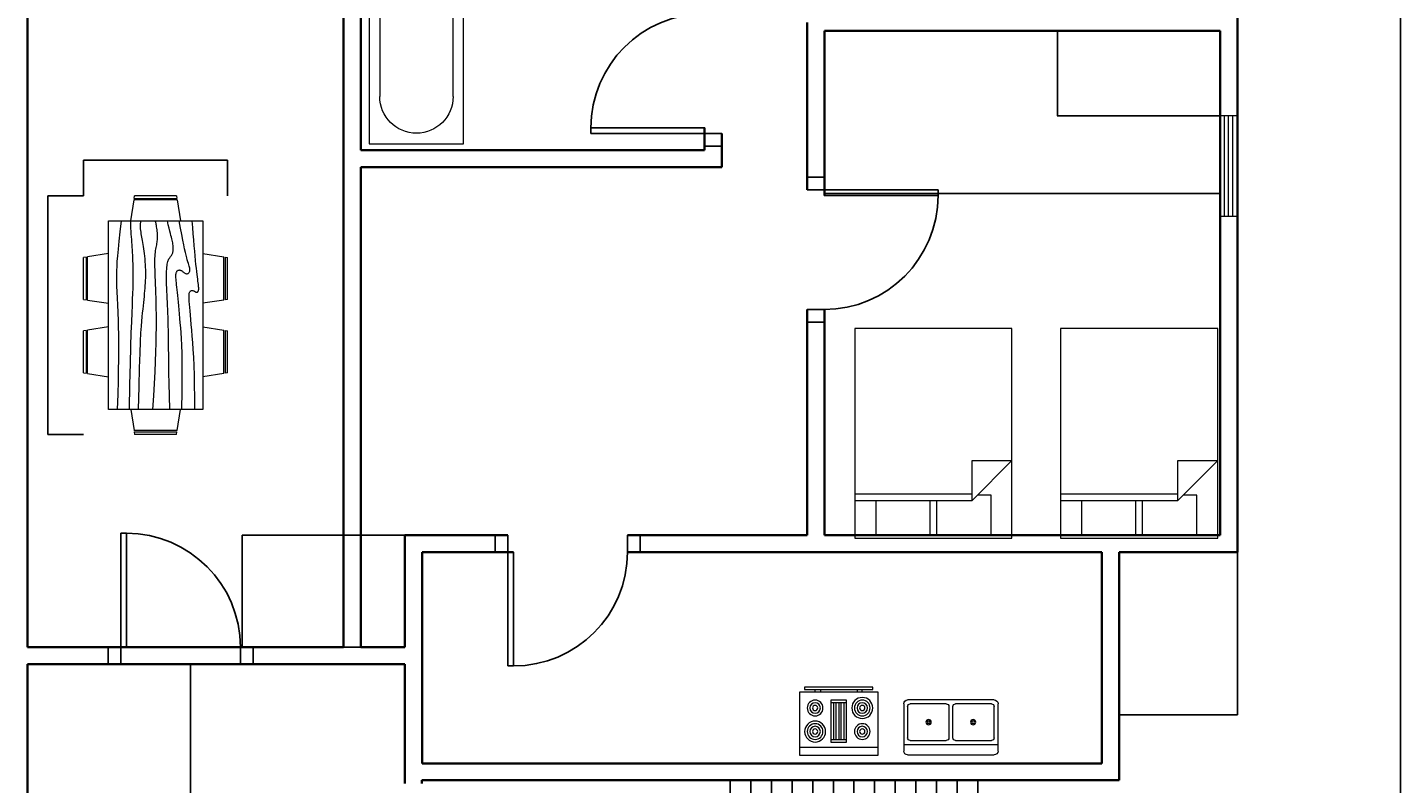
# Model space of a CAD drawing. Units: millimetres. Extents: x 31 to 27050, y -916 to 32407.
# Tile 7 of 7: x 13741 to 27050, y 16782 to 24108. Entities that reach past the tile are written whole.
import ezdxf

# ---------------------------------------------------------------- set-up
doc = ezdxf.new("R2010")
doc.units = ezdxf.units.MM
for name, color, linetype, lineweight in [('A-ANNO-DIMS', 2, 'Continuous', 18), ('A-DOOR', 3, 'Continuous', 25), ('A-EQPM', 8, 'Continuous', 18), ('A-FLOR-FIXT', 9, 'Continuous', 18), ('A-FLOR-STRS', 7, 'Continuous', 25), ('A-FURN', 8, 'Continuous', 13), ('A-GLAZ', 4, 'Continuous', 18), ('A-WALL', 7, 'Continuous', 35)]:
    doc.layers.add(name, color=color, linetype=linetype, lineweight=lineweight)
doc.styles.get("Standard").update_dxf_attribs({"font": 'arial.ttf'})
doc.dimstyles.get("Standard").update_dxf_attribs({"dimtxt": 0.18, "dimasz": 0.18, "dimexe": 0.18, "dimexo": 0.0625, "dimgap": 0.09, "dimtad": 0, "dimtih": 1, "dimtoh": 1, "dimdec": 4, "dimzin": 0, "dimdsep": 46, "dimtxsty": 'Standard', "dimcen": 0.09, "dimadec": 0, "dimazin": 0, "dimtfac": 1, "dimtdec": 4, "dimtofl": 0, "dimtmove": 0, "dimatfit": 3, "dimfxl": 1, "dimtolj": 1, "dimtzin": 0, "dimarcsym": 0})

# ---------------------------------------------------------------- blocks, each defined once
blk = doc.blocks.new('Dining Set - 36 x 72 in.')
for p, q in [((-22, 27.5), (-22.15620000000001, 26.50042)), ((-5.841600000000028, 26.5), (-22.15340000000003, 26.5)), ((-22, 27.5), (-6, 27.5)), ((-5.843700000000012, 26.49966), (-6, 27.5)), ((6, 27.5), (5.843799999999987, 26.50042)), ((22.15839999999997, 26.5), (5.846599999999966, 26.5)), ((6, 27.5), (22, 27.5)), ((22.15629999999999, 26.49966), (22, 27.5)), ((-22.23430000000002, 26.00059), (-23.48470000000003, 17.99762)), ((-22.23040000000003, 26), (-5.760800000000017, 26)), ((-4.515199999999992, 17.99762), (-5.765500000000031, 25.99926)), ((5.765699999999981, 26.00059), (4.515299999999967, 17.99762)), ((5.769599999999968, 26), (22.23919999999998, 26)), ((23.48480000000001, 17.99762), (22.23449999999997, 25.99926)), ((36, 18), (-36, 18)), ((-36, 18), (-36, -18)), ((36, -18), (36, 18)), ((-45.49999999999999, 8.000000000000004), (-44.50040000000001, 8.156170000000007)), ((-45.49999999999999, 8.000000000000004), (-45.49999999999999, -7.999999999999996)), ((-44.5, -8.15843), (-44.5, 8.153380000000002)), ((-44.00060000000002, 8.234280000000002), (-35.99760000000003, 9.484740000000006)), ((-44, 8.230410000000003), (-44, -8.239149999999999)), ((44.00059999999996, 8.234280000000002), (35.99759999999998, 9.484740000000006)), ((44, 8.230410000000003), (44, -8.239149999999999)), ((44.5, -8.15843), (44.5, 8.153380000000002)), ((45.49999999999999, 8.000000000000004), (44.50049999999999, 8.156170000000007)), ((45.49999999999999, 8.000000000000004), (45.49999999999999, -7.999999999999996)), ((-44.49970000000002, -8.156309999999994), (-45.49999999999999, -7.999999999999996)), ((-35.99760000000003, -9.484759999999998), (-43.9993, -8.234499999999993)), ((35.99759999999998, -9.484759999999998), (43.9993, -8.234499999999993)), ((44.49969999999995, -8.156309999999994), (45.49999999999999, -7.999999999999996)), ((-36, -18), (36, -18)), ((-22.23430000000002, -26.0006), (-23.48470000000003, -17.99762)), ((-4.515199999999992, -17.99762), (-5.765500000000031, -25.99928)), ((5.765699999999981, -26.0006), (4.515299999999967, -17.99762)), ((23.48480000000001, -17.99762), (22.23449999999997, -25.99928)), ((-22.23040000000003, -26), (-5.760800000000017, -26)), ((5.769599999999968, -26), (22.23919999999998, -26)), ((-22, -27.5), (-22.15620000000001, -26.50044)), ((-5.841600000000028, -26.5), (-22.15340000000003, -26.5)), ((-22, -27.5), (-6, -27.5)), ((-5.843700000000012, -26.49967), (-6, -27.5)), ((6, -27.5), (5.843799999999987, -26.50044)), ((22.15839999999997, -26.5), (5.846599999999966, -26.5)), ((6, -27.5), (22, -27.5)), ((22.15629999999999, -26.49967), (22, -27.5))]:
    blk.add_line(p, q)
for points in [[(-36, 15), (-31.17720000000003, 14.97754), (-26.80790000000002, 14.91406), (-22.85380000000003, 14.81543), (-19.27600000000001, 14.6875), (-16.03620000000001, 14.53613), (-13.09570000000002, 14.36718), (-10.41590000000002, 14.18652), (-7.958300000000008, 14), (-5.690400000000011, 13.81315), (-3.603499999999996, 13.63021), (-1.695400000000006, 13.45508), (0.0364999999999896, 13.29166), (1.594499999999982, 13.14388), (2.981099999999969, 13.01562), (4.198800000000005, 12.9108), (5.25, 12.83333), (6.139299999999991, 12.78613), (6.880200000000002, 12.76823), (7.488299999999981, 12.77767), (7.979199999999991, 12.8125), (8.368499999999983, 12.87077), (8.671899999999994, 12.95052), (8.904899999999998, 13.0498), (9.083300000000008, 13.16666), (9.220499999999959, 13.29899000000001), (9.32159999999999, 13.44401), (9.389499999999998, 13.59879), (9.427099999999996, 13.76041), (9.437299999999993, 13.92594), (9.423200000000008, 14.09245), (9.387499999999989, 14.257), (9.333300000000008, 14.41666), (9.263800000000003, 14.56917), (9.183600000000013, 14.71484), (9.097499999999968, 14.85465), (9.010400000000004, 14.98958), (8.92719999999997, 15.12060000000001), (8.852899999999975, 15.2487), (8.79219999999998, 15.37483), (8.75, 15.5), (8.730500000000006, 15.62467), (8.734399999999994, 15.74739), (8.761699999999962, 15.86621), (8.8125, 15.97916), (8.886699999999962, 16.08431), (8.984399999999994, 16.17968), (9.105500000000006, 16.26334), (9.25, 16.33333), (9.418900000000008, 16.38802), (9.617199999999968, 16.42708), (9.850599999999986, 16.45052), (10.125, 16.45833), (10.44630000000001, 16.45052), (10.82029999999997, 16.42708), (11.25290000000001, 16.38802), (11.75, 16.33333), (12.3184, 16.26318), (12.96940000000001, 16.17838), (13.7151, 16.07991), (14.5677, 15.96875), (15.53949999999997, 15.84586), (16.64259999999996, 15.71224), (17.88929999999999, 15.56884), (19.29169999999999, 15.41666), (20.85899999999998, 15.25667), (22.58789999999999, 15.08984), (24.47210000000001, 14.91715), (26.5052, 14.73958), (28.68090000000001, 14.5581), (30.99289999999996, 14.3737), (33.43469999999996, 14.18733), (36, 14)], [(-36, 10), (-28.97660000000002, 10.14274000000001), (-23.17250000000001, 10.20442), (-18.42410000000001, 10.19775), (-14.5677, 10.13541), (-11.43990000000002, 10.03011), (-8.87700000000001, 9.894530000000007), (-6.715399999999988, 9.741370000000005), (-4.791699999999991, 9.58333), (-2.96980000000002, 9.43082), (-1.224600000000009, 9.285150000000005), (0.4414999999999623, 9.14534), (2.02600000000001, 9.010410000000004), (3.526599999999973, 8.879390000000004), (4.940799999999967, 8.751300000000004), (6.265999999999962, 8.625160000000005), (7.5, 8.500000000000004), (8.641099999999994, 8.375490000000003), (9.691399999999987, 8.253900000000005), (10.65379999999999, 8.13818), (11.53120000000001, 8.031250000000004), (12.32669999999996, 7.936030000000005), (13.043, 7.85547), (13.68309999999997, 7.792480000000001), (14.25, 7.750000000000003), (14.74709999999999, 7.730300000000003), (15.17969999999997, 7.733070000000001), (15.55369999999999, 7.757320000000003), (15.875, 7.80208), (16.14940000000001, 7.866370000000006), (16.38279999999997, 7.94922), (16.58109999999999, 8.04964), (16.75, 8.166660000000004), (16.89439999999996, 8.29915), (17.01429999999999, 8.445310000000003), (17.1089, 8.603190000000001), (17.17709999999999, 8.77083), (17.21799999999996, 8.946290000000001), (17.2305, 9.127600000000005), (17.21369999999996, 9.312820000000006), (17.16669999999999, 9.500000000000004), (17.08949999999999, 9.687500000000004), (16.98699999999996, 9.875000000000004), (16.86489999999998, 10.0625), (16.72919999999999, 10.25), (16.5856, 10.4375), (16.44009999999997, 10.625), (16.29849999999999, 10.8125), (16.16669999999999, 11), (16.05000000000001, 11.18733), (15.95179999999999, 11.3737), (15.8752, 11.5581), (15.8229, 11.73958), (15.798, 11.91715), (15.80340000000001, 12.08984), (15.84199999999998, 12.25667), (15.91669999999999, 12.41666), (16.02949999999998, 12.56836), (16.17840000000001, 12.70833), (16.3605, 12.83268), (16.5729, 12.9375), (16.8127, 13.01888000000001), (17.07679999999999, 13.07291), (17.36250000000001, 13.0957), (17.66669999999999, 13.08333), (17.98939999999999, 13.03312), (18.34179999999998, 12.94726), (18.7382, 12.82918), (19.1927, 12.68229), (19.71949999999998, 12.51001), (20.33269999999999, 12.31575), (21.04649999999998, 12.10294), (21.875, 11.875), (22.83569999999997, 11.63354), (23.95900000000001, 11.37304), (25.27859999999999, 11.08618), (26.82819999999998, 10.76562), (28.64139999999998, 10.40405), (30.75200000000001, 9.994140000000005), (33.1936, 9.528560000000002), (36, 9.000000000000004)], [(-36, 5.500000000000003), (-30.71570000000003, 5.334800000000004), (-26.06900000000002, 5.20963), (-21.99459999999999, 5.11767), (-18.42709999999999, 5.05208), (-15.30090000000001, 5.006020000000003), (-12.55080000000004, 4.972650000000005), (-10.1112, 4.945150000000001), (-7.916699999999991, 4.916660000000003), (-5.908999999999991, 4.881670000000003), (-4.058600000000012, 4.839840000000005), (-2.342899999999985, 4.792150000000003), (-0.7395999999999959, 4.73958), (0.7738999999999692, 4.683100000000006), (2.21999999999997, 4.623700000000003), (3.621299999999962, 4.562330000000006), (5, 4.500000000000003), (6.37299999999999, 4.437820000000005), (7.734399999999993, 4.377600000000004), (9.072299999999984, 4.321290000000001), (10.375, 4.27083), (11.63089999999999, 4.228190000000001), (12.8281, 4.195310000000002), (13.95509999999996, 4.17415), (15, 4.166660000000003), (15.95400000000001, 4.174480000000006), (16.81899999999996, 4.197910000000003), (17.6001, 4.236980000000006), (18.30209999999999, 4.291660000000003), (18.92989999999997, 4.361980000000006), (19.48829999999998, 4.447910000000003), (19.98230000000001, 4.549480000000006), (20.41669999999999, 4.666660000000003), (20.79689999999999, 4.798990000000006), (21.1302, 4.944010000000002), (21.42449999999997, 5.098790000000004), (21.6875, 5.260410000000003), (21.92709999999999, 5.42594), (22.15109999999999, 5.592450000000003), (22.36719999999997, 5.757000000000001), (22.58339999999998, 5.916660000000003), (22.80649999999997, 6.068680000000004), (23.04039999999998, 6.210930000000001), (23.28789999999998, 6.341470000000004), (23.5521, 6.45833), (23.83580000000001, 6.559570000000004), (24.142, 6.643230000000006), (24.4735, 6.707350000000001), (24.83339999999998, 6.750000000000003), (25.2235, 6.76969), (25.642, 6.766920000000002), (26.08580000000001, 6.74267), (26.5521, 6.697910000000003), (27.03789999999998, 6.633620000000004), (27.54039999999998, 6.550780000000006), (28.05649999999997, 6.450360000000006), (28.58339999999998, 6.33333), (29.12419999999997, 6.19987), (29.70709999999997, 6.046870000000001), (30.36609999999996, 5.870440000000005), (31.1354, 5.666660000000003), (32.04929999999996, 5.431640000000005), (33.142, 5.161460000000001), (34.44749999999999, 4.852210000000003), (36, 4.500000000000003)], [(-36, -0.9999999999999964), (-30.79150000000004, -0.6590999999999987), (-26.01949999999999, -0.3821599999999954), (-21.65190000000001, -0.1628399999999992), (-17.65629999999999, 0.0052100000000017), (-14.00049999999999, 0.1283300000000018), (-10.65230000000002, 0.2128900000000051), (-7.579600000000027, 0.2652200000000029), (-4.75, 0.2916600000000038), (-2.134000000000014, 0.2979300000000045), (0.2878000000000043, 0.287110000000002), (2.5317, 0.2616300000000002), (4.614599999999995, 0.2239600000000017), (6.552899999999965, 0.1765100000000039), (8.363299999999981, 0.1217400000000062), (10.06229999999999, 0.0620900000000013), (11.66669999999999, 3.6e-15), (13.18989999999996, -0.0620099999999972), (14.63409999999999, -0.1210999999999949), (15.9982, -0.174319999999998), (17.28129999999999, -0.2187499999999964), (18.48230000000001, -0.2514699999999941), (19.6003, -0.2695299999999996), (20.6343, -0.2700199999999988), (21.58339999999999, -0.2499999999999964), (22.44810000000001, -0.2076799999999999), (23.23570000000001, -0.1458399999999962), (23.95490000000001, -0.0683599999999949), (24.6146, 0.0208300000000001), (25.2235, 0.1178400000000046), (25.79039999999998, 0.2187500000000035), (26.32409999999999, 0.3196600000000025), (26.83339999999998, 0.4166600000000038), (27.32650000000001, 0.5061800000000041), (27.80989999999997, 0.5859300000000012), (28.2894, 0.6539700000000046), (28.77089999999999, 0.7083300000000002), (29.26009999999997, 0.7470700000000045), (29.76299999999998, 0.7682300000000062), (30.28550000000001, 0.7698500000000017), (30.83339999999998, 0.7500000000000036), (31.40879999999999, 0.707840000000001), (31.99939999999998, 0.6471300000000006), (32.589, 0.5727500000000028), (33.16149999999999, 0.4895800000000002), (33.70079999999996, 0.402500000000007), (34.19079999999997, 0.3164000000000051), (34.61529999999999, 0.2361600000000017), (34.95839999999998, 0.1666600000000038), (35.20990000000001, 0.1116500000000009), (35.38479999999998, 0.0703100000000028), (35.50399999999996, 0.0406900000000015), (35.58859999999999, 0.0208300000000001), (35.65940000000001, 0.0087900000000012), (35.73769999999996, 0.0026000000000046), (35.8442, 0.0003200000000056), (36, 3.6e-15)], [(-36, -6.499999999999996), (-27.18430000000001, -6.312669999999993), (-20.084, -6.126299999999996), (-14.46899999999999, -5.941899999999993), (-10.10939999999999, -5.760419999999999), (-6.77520000000004, -5.582849999999996), (-4.236300000000028, -5.410159999999994), (-2.262900000000001, -5.243329999999996), (-0.625, -5.083339999999996), (0.8707999999999742, -4.930989999999997), (2.271500000000003, -4.786459999999994), (3.587199999999995, -4.649739999999997), (4.828100000000006, -4.520839999999996), (6.004599999999982, -4.399739999999997), (7.127000000000009, -4.286459999999994), (8.205299999999966, -4.180989999999997), (9.25, -4.083339999999996), (10.27049999999997, -3.993819999999995), (11.27339999999998, -3.914069999999998), (12.2647, -3.846029999999995), (13.25, -3.791669999999999), (14.23539999999997, -3.752929999999995), (15.22659999999996, -3.731769999999993), (16.22949999999997, -3.730149999999998), (17.25, -3.749999999999996), (18.2912, -3.792479999999994), (19.3451, -3.855469999999993), (20.40089999999998, -3.936039999999994), (21.4479, -4.031249999999996), (22.47539999999998, -4.138189999999998), (23.47269999999998, -4.253909999999994), (24.4289, -4.375489999999995), (25.33339999999999, -4.499999999999996), (26.17849999999999, -4.624919999999999), (26.96940000000001, -4.749349999999996), (27.71449999999999, -4.872809999999997), (28.4219, -4.994789999999998), (29.09999999999996, -5.114829999999994), (29.75720000000001, -5.232419999999994), (30.40159999999997, -5.347089999999997), (31.04169999999999, -5.458339999999996), (31.68369999999999, -5.564369999999993), (32.32619999999997, -5.658209999999993), (32.9658, -5.731529999999995), (33.59899999999999, -5.776039999999998), (34.22239999999999, -5.783449999999998), (34.83269999999999, -5.745449999999994), (35.4264, -5.653729999999999), (36, -5.499999999999996)], [(-36, -9.999999999999996), (-26.40219999999999, -9.812989999999996), (-18.46750000000003, -9.628909999999994), (-11.9839, -9.450689999999998), (-6.739599999999995, -9.281249999999996), (-2.522600000000011, -9.123539999999995), (0.8788999999999872, -8.980469999999993), (3.676899999999989, -8.854979999999994), (6.083300000000008, -8.749999999999996), (8.276700000000005, -8.667649999999998), (10.30209999999999, -8.606769999999994), (12.1712, -8.565429999999996), (13.89580000000001, -8.54167), (15.48759999999998, -8.533529999999995), (16.95830000000001, -8.539069999999999), (18.31970000000001, -8.556319999999994), (19.58339999999998, -8.583339999999996), (20.76159999999999, -8.618409999999994), (21.86849999999998, -8.660809999999994), (22.91879999999998, -8.710039999999996), (23.9271, -8.765629999999998), (24.90809999999999, -8.827069999999996), (25.87629999999996, -8.89388), (26.84649999999999, -8.96558), (27.83339999999999, -9.04167), (28.84739999999999, -9.121179999999997), (29.88279999999998, -9.201169999999994), (30.93000000000001, -9.278239999999993), (31.97919999999999, -9.348959999999995), (33.02049999999997, -9.409909999999998), (34.04429999999996, -9.45768), (35.04069999999996, -9.488849999999996), (36, -9.499999999999996)], [(-36, -14.5), (-30.0881, -14.33512999999999), (-25.03320000000002, -14.21224), (-20.7312, -14.12646999999999), (-17.0781, -14.07292), (-13.97000000000003, -14.04670999999999), (-11.30270000000001, -14.04296999999999), (-8.972399999999993, -14.05680999999999), (-6.875, -14.08333999999999), (-4.922400000000038, -14.11832999999999), (-3.09050000000002, -14.16015999999999), (-1.370900000000006, -14.20784999999999), (0.2447999999999979, -14.26042), (1.764700000000004, -14.31689999999999), (3.197299999999984, -14.37629999999999), (4.550700000000006, -14.43766999999999), (5.833300000000008, -14.5), (7.055399999999963, -14.5621), (8.235000000000014, -14.62174999999999), (9.392200000000003, -14.67652), (10.54689999999999, -14.72395999999999), (11.7192, -14.76164), (12.92899999999997, -14.78711), (14.19649999999996, -14.79794), (15.54169999999999, -14.79167), (16.99329999999998, -14.76423999999999), (18.61519999999996, -14.70508), (20.48039999999998, -14.60197), (22.66149999999999, -14.44270999999999), (25.2312, -14.21509), (28.26240000000002, -13.90689999999999), (31.8277, -13.50594), (36, -13)]]:
    blk.add_lwpolyline(points)
blk = doc.blocks.new('Range-Oven - 30 in top')
for p, q in [((0, -3), (30, -3)), ((12, -6), (18, -6)), ((13, -19.999996), (13, -6)), ((14, -6), (14, -19.999996)), ((15, -19.999996), (15, -6)), ((16, -6), (16, -19.999996)), ((17, -19.999996), (17, -6)), ((18, -19.999996), (12, -19.999996)), ((6.000000000000003, -23.99999600000001), (6.000000000000003, -24.999996)), ((8.000000000000004, -24.999996), (8.000000000000004, -23.99999600000001)), ((22.00000000000001, -24.999996), (22.00000000000001, -23.99999600000001)), ((24, -23.99999600000001), (24, -24.999996))]:
    blk.add_line(p, q)
for points in [[(0, -23.99999600000001), (0, 0), (30, 0), (30, -23.99999600000001)], [(12, -20.999996), (12, -5), (18, -5), (18, -20.999996)], [(2.000000000000003, -25.999996), (2.000000000000003, -24.999996), (28.00000000000001, -24.999996), (28.00000000000001, -25.999996)]]:
    blk.add_lwpolyline(points, close=True)
for centre, radius in [((6.000000000000003, -9.0000002), 4), ((6.000000000000003, -9.0000002), 3), ((6.000000000000003, -9.0000002), 2), ((6.000000000000003, -9.0000002), 1), ((24, -9.0000002), 3), ((24, -9.0000002), 2), ((24, -9.0000002), 1), ((6.000000000000003, -18), 3), ((24, -18), 4), ((24, -18), 3), ((6.000000000000003, -18), 2), ((6.000000000000003, -18), 1), ((24, -18), 2), ((24, -18), 1)]:
    blk.add_circle(centre, radius)
blk = doc.blocks.new('Sink-double - 36 in top')
for p, q in [((-18, -4), (18, -4)), ((-0.75, -18.5), (-0.75, -6.5)), ((0.75, -6.5), (0.75, -18.5))]:
    blk.add_line(p, q)
for points in [[(-16.5, 0), (16.5, 0)], [(-18, -19.5), (-18, -1.5)], [(18, -1.5), (18, -19.5)], [(-16.5, -18.5), (-16.5, -6.5)], [(-15.5, -5.5), (-1.75, -5.5)], [(1.75, -5.5), (15.5, -5.5)], [(16.5, -6.5), (16.5, -18.5)], [(-1.75, -19.5), (-15.5, -19.5)], [(15.5, -19.5), (1.75, -19.5)], [(16.5, -21), (-16.5, -21)]]:
    blk.add_lwpolyline(points)
for centre, radius in [((-8.5, -12.5), 1), ((-8.5, -12.5), 0.5), ((8.5, -12.5), 1), ((8.5, -12.5), 0.5)]:
    blk.add_circle(centre, radius)
for centre, radius, start, end in [((-16.5, -1.5), 1.5, 90, 180), ((16.5, -1.5), 1.5, 0, 90), ((-15.5, -6.5), 1, 90, 180), ((-1.75, -6.5), 1, 0, 90), ((1.75, -6.5), 1, 90, 180), ((15.5, -6.5), 1, 0, 90), ((-16.5, -19.5), 1.5, 180, 270), ((-15.5, -18.5), 1, 180, 270), ((-1.75, -18.5), 1, 270, 0), ((1.75, -18.5), 1, 180, 270), ((15.5, -18.5), 1, 270, 0), ((16.5, -19.5), 1.5, 270, 0)]:
    blk.add_arc(centre, radius, start, end)
blk = doc.blocks.new('Bath Tub - 26 x 60 in.')
for p, q in [((8, -18), (10, -18)), ((9, -17), (9, -19))]:
    blk.add_line(p, q)
blk.add_lwpolyline([(0, -36), (0, 0), (60, 0), (60, -36)], close=True)
for points in [[(6, -4), (42, -4)], [(4, -30), (4, -6)], [(42, -32), (6, -32)]]:
    blk.add_lwpolyline(points)
for radius in [1.5, 1]:
    blk.add_circle((9, -18), radius)
for centre, radius, start, end in [((5.75, -5.75), 1.767766999999999, 81.86989999999999, 188.1301), ((42, -18), 14, 270, 90), ((5.75, -30.25), 1.767766999999999, 171.8699, 278.1301)]:
    blk.add_arc(centre, radius, start, end)
blk = doc.blocks.new('Bed - Queen')
for p, q in [((0, -80.00003000000002), (0, 0)), ((0, 0), (59.99998999999999, 0)), ((59.99998999999999, 0), (59.99998999999999, -80.00003000000002)), ((7.99999, -1.200000000000017), (28.79998, -1.200000000000017)), ((7.99999, -14.4), (7.99999, -1.200000000000017)), ((28.79998, -1.200000000000017), (28.79998, -14.4)), ((31.19999, -1.200000000000017), (51.99999000000001, -1.200000000000017)), ((31.19999, -14.4), (31.19999, -1.200000000000017)), ((51.99999000000001, -1.200000000000017), (51.99999000000001, -16.4)), ((0, -14.4), (44.79999999999999, -14.4)), ((59.99998999999999, -29.60000000000001), (44.79999999999999, -14.4)), ((44.79999999999999, -14.4), (44.79999999999999, -29.60000000000001)), ((44.79999999999999, -16.80000000000001), (0, -16.80000000000001)), ((51.99999000000001, -16.4), (46.79936, -16.4)), ((44.79999999999999, -29.60000000000001), (59.99998999999999, -29.60000000000001)), ((59.99998999999999, -80.00003000000002), (0, -80.00003000000002))]:
    blk.add_line(p, q)
blk = doc.blocks.new('Window - Wood Frame 36 in. Wide plan')
for p, q in [((0, 6), (0, 0)), ((36, 6), (36, 0)), ((0, 4.5), (36, 4.5)), ((0, 3), (36, 3)), ((0, 1.5), (36, 1.5))]:
    blk.add_line(p, q)
blk = doc.blocks.new('DOOR-SINGLE-1104')
for p, q in [((56.41678681898429, 1104.337341461596), (-7.18501e-11, 1104.337341461596)), ((-7.18501e-11, 1104.337341461596), (-7.18501e-11, 3.638e-12)), ((56.41678681898429, 7.276e-12), (56.41678681898429, 1104.337341461596)), ((-1226.913698425656, -163.8831223050438), (-1226.913698425656, 3.638e-12)), ((-1104.337341461589, 3.638e-12), (-1226.913698425656, 7.276e-12)), ((-1104.337341461589, 3.638e-12), (-1104.337341461589, -163.8831223050438)), ((-7.18501e-11, 3.638e-12), (56.41678681898429, 7.276e-12)), ((56.41678681898429, -163.8831223050438), (56.41678681898429, 3.638e-12)), ((56.41678681898429, 3.638e-12), (178.9931437830519, 3.638e-12)), ((178.9931437830519, 3.638e-12), (178.9931437830519, -163.8831223050438)), ((-1104.337341461589, -163.8831223050438), (-1226.913698425656, -163.8831223050438)), ((178.9931437830519, -163.8831223050438), (56.41678681898429, -163.8831223050438))]:
    blk.add_line(p, q)
blk.add_arc((0, 3.638e-12), 1104.337341461589, 90, 180)
blk = doc.blocks.new('STAIR-RETURN-2400')
for p, q in [((9.095e-13, 2345.636859649549), (9.095e-13, -1.819e-12)), ((200.0000000000009, 2345.636859649549), (200.0000000000009, -1.819e-12)), ((400.0000000000008, 2345.636859649549), (400.0000000000008, -1.819e-12)), ((600.0000000000008, 2345.636859649549), (600.0000000000008, -1.819e-12)), ((800.0000000000008, 2345.636859649552), (800.0000000000008, 1.819e-12)), ((1000.000000000001, 2345.636859649556), (1000.000000000001, 5.457e-12)), ((1200.000000000001, 2345.636859649556), (1200.000000000001, 5.457e-12)), ((1400.000000000001, 2345.636859649556), (1400.000000000001, 5.457e-12)), ((1600.000000000001, 2345.636859649559), (1600.000000000001, 9.0949e-12)), ((1800.000000000001, 2345.636859649559), (1800.000000000001, 9.0949e-12)), ((2000.000000000001, 2345.636859649559), (2000.000000000001, 9.0949e-12)), ((2200.000000000001, 2345.636859649563), (2200.000000000001, 1.27329e-11)), ((2400.000000000001, 2345.636859649563), (2400.000000000001, 1.27329e-11)), ((-415.9249645337103, 697.4958917418807), (-415.9249645337103, 1817.654410237617)), ((-415.9249645337103, 1817.654410237617), (2588.331988211024, 1817.654410237617)), ((9.095e-13, 1172.818429824772), (9.095e-13, 1272.818429824772)), ((9.095e-13, 1272.818429824772), (2400.000000000001, 1272.818429824774)), ((2400.000000000001, 1272.818429824774), (2400.000000000001, 1072.818429824774)), ((2400.000000000001, 1072.818429824774), (9.095e-13, 1072.818429824774)), ((2597.09055342863, 697.4958917418807), (-415.9249645337103, 697.4958917418807))]:
    blk.add_line(p, q)
blk.add_lwpolyline([(2948.607295106225, 1817.654410237617), (2588.331988211024, 2025.65945565594), (2588.331988211024, 1609.649364819299)], close=True)
blk = doc.blocks.new('*D28')
at = {"layer": 'A-ANNO-DIMS', "color": 0, "lineweight": -2, "transparency": 16777216}
for p, q in [((14283.95080415747, 22476.21173650058), (13937.12330415747, 22476.21173650058)), ((13937.30330415747, 22476.03173650058), (13937.30330415747, 21320.6948674692)), ((13937.30330415747, 20164.99173650058), (13937.30330415747, 21320.32860553196)), ((14283.95080415747, 20164.81173650058), (13937.12330415747, 20164.81173650058))]:
    blk.add_line(p, q, dxfattribs=at)
at = {"layer": 'A-ANNO-DIMS', "color": 0, "transparency": 16777216}
for points in [[(13937.27330415747, 22476.03173650058), (13937.33330415747, 22476.03173650058), (13937.30330415747, 22476.21173650058)], [(13937.27330415747, 20164.99173650058), (13937.33330415747, 20164.99173650058), (13937.30330415747, 20164.81173650058)]]:
    blk.add_solid(points, dxfattribs=at)
at = {"layer": 'Defpoints', "color": 0, "transparency": 16777216}
for p in [(13937.30330415747, 22476.21173650058), (14284.01330415747, 22476.21173650058), (14284.01330415747, 20164.81173650058)]:
    blk.add_point(p, dxfattribs=at)
at = {"layer": 'A-ANNO-DIMS', "color": 0, "transparency": 16777216, "insert": (13937.30330415747, 21320.51173650057), "char_height": 0.18, "attachment_point": 5}
blk.add_mtext('\\A1;DINING SET 2311 TYP.', dxfattribs=at)
blk = doc.blocks.new('*D29')
at = {"layer": 'A-ANNO-DIMS', "color": 0, "lineweight": -2, "transparency": 16777216}
for p, q in [((14284.01330415746, 22476.27423650057), (14284.01330415746, 22823.10173650057)), ((14284.19330415746, 22822.92173650057), (14981.85383621749, 22822.92173650057)), ((15680.83330415746, 22822.92173650057), (14983.17277209743, 22822.92173650057)), ((15681.01330415746, 22476.27423650057), (15681.01330415746, 22823.10173650057))]:
    blk.add_line(p, q, dxfattribs=at)
at = {"layer": 'A-ANNO-DIMS', "color": 0, "transparency": 16777216}
for points in [[(14284.19330415746, 22822.95173650057), (14284.19330415746, 22822.89173650057), (14284.01330415746, 22822.92173650057)], [(15680.83330415746, 22822.95173650057), (15680.83330415746, 22822.89173650057), (15681.01330415746, 22822.92173650057)]]:
    blk.add_solid(points, dxfattribs=at)
at = {"layer": 'Defpoints', "color": 0, "transparency": 16777216}
for p in [(15681.01330415746, 22822.92173650057), (14284.01330415746, 22476.21173650057), (15681.01330415746, 22476.21173650057)]:
    blk.add_point(p, dxfattribs=at)
at = {"layer": 'A-ANNO-DIMS', "color": 0, "transparency": 16777216, "insert": (14982.51330415746, 22822.92173650057), "char_height": 0.18, "attachment_point": 5}
blk.add_mtext('\\A1;1397 TYP.', dxfattribs=at)
blk = doc.blocks.new('*D47')
at = {"layer": 'A-ANNO-DIMS', "color": 0, "lineweight": -2, "transparency": 16777216}
for p, q in [((25471.21116800002, 30827.53125900001), (27050.32866800003, 30827.53125900001)), ((27050.14866800003, 30827.35125900001), (27050.14866800003, 15745.77166202933)), ((27050.14866800004, 663.8281360000004), (27050.14866800003, 15745.40773297067)), ((25471.21116800002, 663.6481360000002), (27050.32866800003, 663.6481360000004))]:
    blk.add_line(p, q, dxfattribs=at)
at = {"layer": 'A-ANNO-DIMS', "color": 0, "transparency": 16777216}
for points in [[(27050.11866800003, 30827.35125900001), (27050.17866800003, 30827.35125900001), (27050.14866800003, 30827.53125900001)], [(27050.11866800004, 663.8281360000004), (27050.17866800004, 663.8281360000004), (27050.14866800004, 663.6481360000004)]]:
    blk.add_solid(points, dxfattribs=at)
at = {"layer": 'Defpoints', "color": 0, "transparency": 16777216}
for p in [(25471.14866800002, 30827.53125900001), (27050.14866800003, 30827.53125900001), (25471.14866800002, 663.6481360000002)]:
    blk.add_point(p, dxfattribs=at)
at = {"layer": 'A-ANNO-DIMS', "color": 0, "transparency": 16777216, "insert": (27050.14866800003, 15745.58969749999), "char_height": 0.18, "attachment_point": 5}
blk.add_mtext('\\A1;30164', dxfattribs=at)
blk = doc.blocks.new('*D60')
at = {"layer": 'A-ANNO-DIMS', "color": 0, "lineweight": -2, "transparency": 16777216}
for p, q in [((21467.81364, 24076.690068), (21467.81363999999, 22497.57256800001)), ((25302.798017, 24076.690068), (25302.79801699999, 22497.57256799999)), ((21467.99364, 22497.752568), (23384.94644241541, 22497.752568)), ((25302.618017, 22497.752568), (23385.66521458458, 22497.752568))]:
    blk.add_line(p, q, dxfattribs=at)
at = {"layer": 'A-ANNO-DIMS', "color": 0, "transparency": 16777216}
for points in [[(21467.99364, 22497.782568), (21467.99364, 22497.722568), (21467.81363999999, 22497.752568)], [(25302.618017, 22497.78256799999), (25302.618017, 22497.722568), (25302.79801699999, 22497.752568)]]:
    blk.add_solid(points, dxfattribs=at)
at = {"layer": 'Defpoints', "color": 0, "transparency": 16777216}
for p in [(21467.81364, 24076.752568), (25302.798017, 24076.752568), (21467.81363999999, 22497.752568)]:
    blk.add_point(p, dxfattribs=at)
at = {"layer": 'A-ANNO-DIMS', "color": 0, "transparency": 16777216, "insert": (23385.30582849999, 22497.752568), "char_height": 0.18, "attachment_point": 5}
blk.add_mtext('\\A1;3835', dxfattribs=at)
blk = doc.blocks.new('*D67')
at = {"layer": 'A-ANNO-DIMS', "color": 0, "lineweight": -2, "transparency": 16777216}
for p, q in [((13740.64783300001, 17938.12750700001), (15319.76533300001, 17938.12750700001)), ((15319.58533300001, 17937.94750700001), (15319.58533300001, 15520.25103252934)), ((15319.58533300001, 13102.19062900001), (15319.58533300001, 15519.88710347067)), ((13740.64783300001, 13102.01062900001), (15319.76533300001, 13102.01062900001))]:
    blk.add_line(p, q, dxfattribs=at)
at = {"layer": 'A-ANNO-DIMS', "color": 0, "transparency": 16777216}
for points in [[(15319.55533300001, 17937.94750700001), (15319.61533300001, 17937.94750700001), (15319.58533300001, 17938.12750700001)], [(15319.55533300001, 13102.19062900001), (15319.61533300001, 13102.19062900001), (15319.58533300001, 13102.01062900001)]]:
    blk.add_solid(points, dxfattribs=at)
at = {"layer": 'Defpoints', "color": 0, "transparency": 16777216}
for p in [(13740.58533300001, 17938.12750700001), (13740.58533300001, 13102.01062900001), (15319.58533300001, 13102.01062900001)]:
    blk.add_point(p, dxfattribs=at)
at = {"layer": 'A-ANNO-DIMS', "color": 0, "transparency": 16777216, "insert": (15319.58533300002, 15520.069068), "char_height": 0.18, "attachment_point": 5}
blk.add_mtext('\\A1;4836', dxfattribs=at)
blk = doc.blocks.new('*D71')
at = {"layer": 'A-ANNO-DIMS', "color": 0, "lineweight": -2, "transparency": 16777216}
for p, q in [((17399.426108, 19189.318846), (15820.30860800001, 19189.318846)), ((15820.48860800001, 19189.138846), (15820.48860800001, 18645.84670202934)), ((15820.48860800001, 18102.190629), (15820.48860800001, 18645.48277297067)), ((17399.426108, 18102.01062900001), (15820.30860800001, 18102.01062900001))]:
    blk.add_line(p, q, dxfattribs=at)
at = {"layer": 'A-ANNO-DIMS', "color": 0, "transparency": 16777216}
for points in [[(15820.45860800001, 19189.138846), (15820.51860800001, 19189.138846), (15820.48860800001, 19189.318846)], [(15820.45860800001, 18102.190629), (15820.51860800001, 18102.190629), (15820.48860800001, 18102.01062900001)]]:
    blk.add_solid(points, dxfattribs=at)
at = {"layer": 'Defpoints', "color": 0, "transparency": 16777216}
for p in [(15820.48860800001, 19189.318846), (17399.48860800001, 19189.318846), (17399.48860800001, 18102.01062900001)]:
    blk.add_point(p, dxfattribs=at)
at = {"layer": 'A-ANNO-DIMS', "color": 0, "transparency": 16777216, "insert": (15820.48860800001, 18645.6647375), "char_height": 0.18, "attachment_point": 5}
blk.add_mtext('\\A1;1087.3', dxfattribs=at)
blk = doc.blocks.new('*D81')
at = {"layer": 'A-ANNO-DIMS', "color": 0, "lineweight": -2, "transparency": 16777216}
for p, q in [((25302.73551700001, 24076.75256800001), (23723.61801700002, 24076.75256800001)), ((23723.79801700001, 24076.572568), (23723.79801700001, 23665.00639602934)), ((23723.79801700001, 23253.07629500001), (23723.79801700001, 23664.64246697067)), ((25302.73551700001, 23252.89629500001), (23723.61801700002, 23252.896295))]:
    blk.add_line(p, q, dxfattribs=at)
at = {"layer": 'A-ANNO-DIMS', "color": 0, "transparency": 16777216}
for points in [[(23723.76801700002, 24076.572568), (23723.82801700001, 24076.572568), (23723.79801700001, 24076.75256800001)], [(23723.76801700002, 23253.07629500001), (23723.82801700001, 23253.07629500001), (23723.79801700001, 23252.896295)]]:
    blk.add_solid(points, dxfattribs=at)
at = {"layer": 'Defpoints', "color": 0, "transparency": 16777216}
for p in [(23723.79801700001, 24076.75256800001), (25302.79801700002, 24076.75256800001), (25302.79801700002, 23252.89629500001)]:
    blk.add_point(p, dxfattribs=at)
at = {"layer": 'A-ANNO-DIMS', "color": 0, "transparency": 16777216, "insert": (23723.79801700001, 23664.8244315), "char_height": 0.18, "attachment_point": 5}
blk.add_mtext('\\A1;823.9', dxfattribs=at)
blk = doc.blocks.new('*D87')
at = {"layer": 'A-ANNO-DIMS', "color": 0, "lineweight": -2, "transparency": 16777216}
for p, q in [((24323.82983, 19025.373224), (24323.82983, 17446.255724)), ((25471.148668, 19025.373224), (25471.148668, 17446.255724)), ((24324.00983, 17446.435724), (24897.0340921105, 17446.435724)), ((25470.968668, 17446.435724), (24897.9444058895, 17446.435724))]:
    blk.add_line(p, q, dxfattribs=at)
at = {"layer": 'A-ANNO-DIMS', "color": 0, "transparency": 16777216}
for points in [[(24324.00983, 17446.46572399999), (24324.00983, 17446.405724), (24323.82983, 17446.435724)], [(25470.968668, 17446.46572399999), (25470.968668, 17446.405724), (25471.148668, 17446.435724)]]:
    blk.add_solid(points, dxfattribs=at)
at = {"layer": 'Defpoints', "color": 0, "transparency": 16777216}
for p in [(24323.82983, 19025.435724), (25471.148668, 19025.435724), (24323.82983, 17446.435724)]:
    blk.add_point(p, dxfattribs=at)
at = {"layer": 'A-ANNO-DIMS', "color": 0, "transparency": 16777216, "insert": (24897.489249, 17446.435724), "char_height": 0.18, "attachment_point": 5}
blk.add_mtext('\\A1;1147.3', dxfattribs=at)

msp = doc.modelspace()

# ---------------------------------------------------------------- linework, layer by layer
at = {"layer": 'A-WALL'}
for p, q in [((25471.14866810643, 19025.43572389214), (25471.14866810643, 30744.3803777756)), ((25471.14866810643, 30744.38037777559), (25471.14866810643, 19106.16796530105)), ((16971.14866810643, 22919.96829640664), (16971.14866810643, 25117.33256545015)), ((13740.58533261045, 18102.01062910059), (13740.58533261045, 24309.37473914616)), ((16802.79801739574, 18469.90100734673), (16802.79801739574, 24309.37473914615)), ((21299.46298919959, 22535.9107124077), (21299.46298919959, 24157.48480901264)), ((21467.81363991028, 24076.75256760374), (22154.74901097826, 24076.75256760373)), ((21467.81363991028, 22479.49392558864), (21467.81363991028, 24076.75256760374)), ((22235.31234647424, 24076.75256760373), (22154.74901097826, 24076.75256760373)), ((22235.31234647424, 24076.75256760373), (25302.79801739574, 24076.75256760373)), ((25302.79801739574, 19189.3188461972), (25302.79801739574, 24076.75256760373)), ((25302.79801739574, 24076.75256760373), (25302.79801739574, 19189.3188461972)), ((20302.79801739574, 23136.49470547361), (20302.79801739574, 22919.96829640663)), ((20471.14866810643, 23080.07791865456), (20471.14866810643, 22836.8174155105)), ((20302.79801739574, 22919.96829640664), (16971.14866810643, 22919.96829640664)), ((20471.14866810643, 22836.8174155105), (20471.14866810643, 22756.08517410159)), ((20390.58533261046, 22756.08517410159), (16971.14866810643, 22756.08517410159)), ((16971.14866810643, 18469.90100734673), (16971.14866810643, 22756.08517410159)), ((20471.14866810643, 22756.08517410159), (20390.58533261046, 22756.08517410159)), ((21299.46298919959, 19189.31884619719), (21299.46298919959, 21375.15658412713)), ((21467.81363991029, 19189.3188461972), (21467.81363991028, 21375.16562071901)), ((17399.48860787868, 18895.47530332579), (17399.48860787868, 19189.3188461972)), ((17399.48860787868, 19189.3188461972), (17536.51130654554, 19189.3188461972)), ((17487.27592309339, 19189.3188461972), (18396.64783631669, 19189.31884619719)), ((19557.40196459726, 19189.3188461972), (21299.46298919959, 19189.3188461972)), ((21467.81363991028, 19189.3188461972), (25302.79801739574, 19189.3188461972)), ((17567.83925858937, 19025.43572389214), (18453.06462313574, 19025.43572389214)), ((17567.83925858938, 18895.47530332579), (17567.83925858937, 19025.43572389215)), ((19557.40196459726, 19025.43572389214), (24155.47917882185, 19025.43572389214)), ((24155.47917882185, 16976.94491866139), (24155.47917882185, 19025.43572389214)), ((24323.82982953254, 19025.43572389214), (25302.79801739574, 19025.43572389214)), ((24323.82982953254, 16976.94491866139), (24323.82982953254, 19025.43572389214)), ((25302.79801739574, 19025.43572389214), (25471.14866810643, 19025.43572389214)), ((17399.48860787868, 18102.0106291006), (17399.48860787868, 18895.47530332579)), ((17567.83925858937, 16976.9449186614), (17567.83925858938, 18895.47530332579)), ((16802.79801739574, 18469.90100734673), (16802.79801739574, 18102.0106291006)), ((16971.14866810643, 18469.90100734673), (16971.14866810643, 18102.0106291006)), ((16802.79801739574, 18102.0106291006), (13740.58533261045, 18102.01062910059)), ((17399.48860787869, 18102.0106291006), (16971.14866810644, 18102.0106291006)), ((13740.58533261045, 13102.01062910059), (13740.58533261045, 17938.12750679554)), ((17399.48860787868, 17938.12750679554), (13740.58533261045, 17938.12750679554)), ((17399.48860787868, 16893.79403776525), (17399.48860787868, 17938.12750679554)), ((24155.47917882185, 16976.94491866139), (17567.83925858937, 16976.9449186614)), ((24323.82982953254, 16976.94491866139), (24323.82982953254, 16813.06179635634)), ((17399.48860787868, 16893.79403776525), (17399.48860787868, 16813.06179635634)), ((17399.48860787868, 16813.06179635634), (17399.48860787868, 16781.90361905769)), ((24323.82982953254, 16813.06179635634), (17563.37173018373, 16813.06179635634)), ((17563.37173018373, 16781.90361905769), (17563.37173018373, 16813.06179635634))]:
    msp.add_line(p, q, dxfattribs=at)

# ---------------------------------------------------------------- block references
at = {"layer": 'A-DOOR', "extrusion": (0, 0, -1), "zscale": -1}
for p, rotation in [((-20307.2655458014, 23136.49470547354), 270.0000000000002), ((-21463.34611150462, 22479.4939255887), 89.99999999999952)]:
    msp.add_blockref('DOOR-SINGLE-1104', p, dxfattribs=dict(at, rotation=rotation))
msp.add_blockref('DOOR-SINGLE-1104', (-14700.67093864094, 18102.01062910057), dxfattribs=at)
at = {"layer": 'A-DOOR', "rotation": 180}
msp.add_blockref('DOOR-SINGLE-1104', (18453.06462313568, 19025.43572389216), dxfattribs=at)
at = {"layer": 'A-EQPM', "xscale": -25.4, "yscale": 25.4, "zscale": 25.4, "rotation": 180}
msp.add_blockref('Range-Oven - 30 in top', (21223.33545355257, 17056.84049659948), dxfattribs=at)
at = {"layer": 'A-FLOR-FIXT', "xscale": -25.4, "yscale": 25.4, "zscale": 25.4}
for name, p, rotation in [('Bath Tub - 26 x 60 in.', (17053.83772899901, 24506.11473923286), 90), ('Sink-double - 36 in top', (22691.66869616197, 17058.95703145353), 180)]:
    msp.add_blockref(name, p, dxfattribs=dict(at, rotation=rotation))
at = {"layer": 'A-FLOR-STRS', "extrusion": (0, 0, -1), "zscale": -1}
msp.add_blockref('STAIR-RETURN-2400', (-22952.576608688, 14467.4249367068), dxfattribs=at)
at = {"layer": 'A-FURN', "xscale": -25.4, "yscale": 25.4, "zscale": 25.4}
for name, p, rotation in [('Dining Set - 36 x 72 in.', (14982.51330415746, 21320.51173650057), 270), ('Bed - Queen', (21760.09753068969, 19158.83884619719), 180), ('Bed - Queen', (23753.99770891948, 19158.8388461972), 180)]:
    msp.add_blockref(name, p, dxfattribs=dict(at, rotation=rotation))
at = {"layer": 'A-GLAZ', "xscale": -27.11229900122799, "yscale": 27.11229900122799, "zscale": 27.11229900122799, "rotation": 270}
msp.add_blockref('Window - Wood Frame 36 in. Wide plan', (25302.79801739574, 22276.8535314434), dxfattribs=at)

# ---------------------------------------------------------------- dimensions: what is measured, and where the dimension line sits
at = {"layer": 'A-ANNO-DIMS'}
for base, p1, p2, angle, override, picture, middle in [((27050.14866800003, 30827.53125900001), (25471.148668, 663.648136), (25471.148668, 30827.531259), 90, {"dimdec": 0, "dimlfac": 1, "dimrnd": 0, "dimzin": 0, "dimdsep": 46, "dimlunit": 2}, '*D47', (27050.14866800003, 15745.58969749999)), ((21467.81363999999, 22497.752568), (25302.798017, 24076.752568), (21467.81364, 24076.752568), 179.9999999999998, {"dimdec": 0, "dimlfac": 1, "dimrnd": 0, "dimzin": 0, "dimdsep": 46, "dimlunit": 2}, '*D60', (23385.30582849999, 22497.752568)), ((23723.79801700001, 24076.75256800001), (25302.798017, 23252.896295), (25302.798017, 24076.752568), 90, {"dimdec": 1, "dimlfac": 1, "dimrnd": 0, "dimzin": 0, "dimdsep": 46, "dimlunit": 2}, '*D81', (23723.79801700001, 23664.8244315)), ((15820.48860800001, 19189.318846), (17399.488608, 18102.010629), (17399.488608, 19189.318846), 90, {"dimdec": 1, "dimlfac": 1, "dimrnd": 0, "dimzin": 0, "dimdsep": 46, "dimlunit": 2}, '*D71', (15820.48860800001, 18645.6647375)), ((24323.82983, 17446.435724), (25471.148668, 19025.435724), (24323.82983, 19025.435724), 180, {"dimdec": 1, "dimlfac": 1, "dimrnd": 0, "dimzin": 0, "dimdsep": 46, "dimlunit": 2}, '*D87', (24897.489249, 17446.435724)), ((15319.58533300001, 13102.01062900001), (13740.585333, 17938.127507), (13740.585333, 13102.010629), 270, {"dimdec": 0, "dimlfac": 1, "dimrnd": 0, "dimzin": 0, "dimdsep": 46, "dimlunit": 2}, '*D67', (15319.58533300002, 15520.069068))]:
    dim = msp.add_linear_dim(base=base, p1=p1, p2=p2, angle=angle, dimstyle='Standard', override=override, dxfattribs=at)
    dim.commit()
    dim.dimension.update_dxf_attribs({"geometry": picture, "text_midpoint": middle})
dim = msp.add_linear_dim(base=(15681.01330415746, 22822.92173650057), p1=(14284.01330415746, 22476.21173650057), p2=(15681.01330415746, 22476.21173650057), text='<> TYP.', dimstyle='Standard', override={"dimdec": 0, "dimlfac": 1, "dimrnd": 0, "dimzin": 0, "dimdsep": 46, "dimlunit": 2}, dxfattribs=at)
dim.commit()
dim.dimension.update_dxf_attribs({"geometry": '*D29', "text_midpoint": (14982.51330415746, 22822.92173650057)})
dim = msp.add_linear_dim(base=(13937.30330415747, 22476.21173650058), p1=(14284.01330415746, 20164.81173650057), p2=(14284.01330415746, 22476.21173650057), angle=90, text='DINING SET <> TYP.', dimstyle='Standard', override={"dimdec": 0, "dimlfac": 1, "dimrnd": 0, "dimzin": 0, "dimdsep": 46, "dimlunit": 2}, dxfattribs=at)
dim.commit()
dim.dimension.update_dxf_attribs({"geometry": '*D28', "text_midpoint": (13937.30330415747, 21320.51173650057)})

doc.saveas('drawing.dxf')
